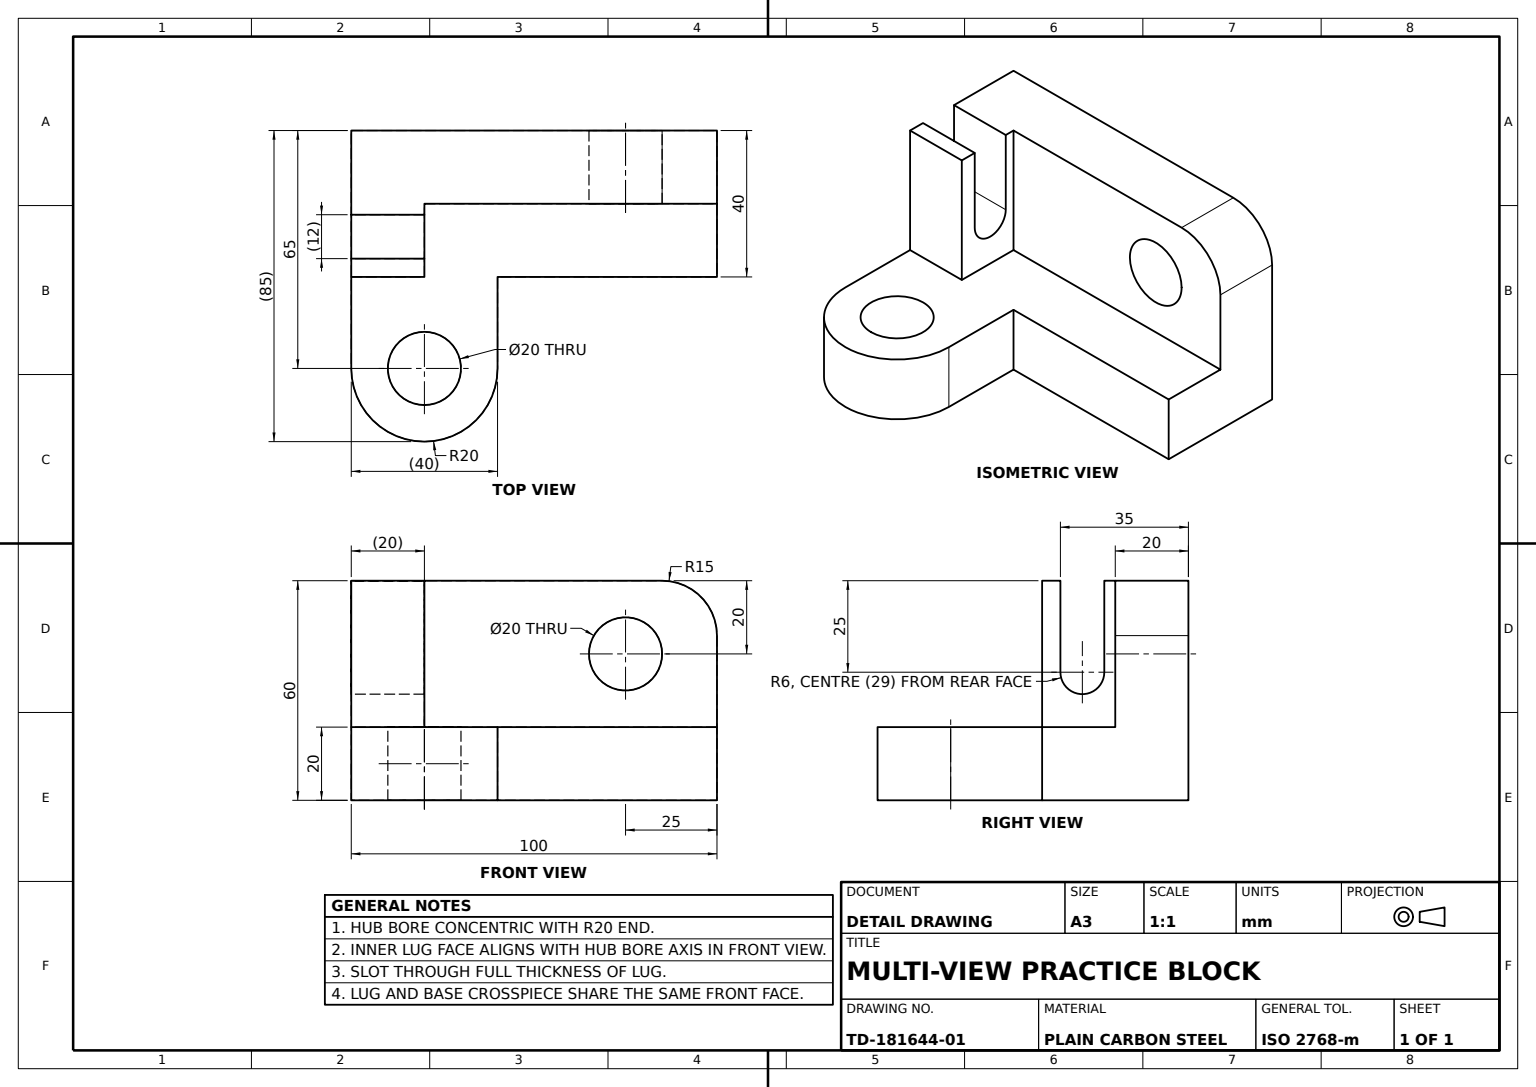
SolidWorks part; units mm, degrees
material "Plain Carbon Steel"
ref_plane "Front Plane" through (0, 0, 0) normal (0, 0, 1) x (1, 0, 0)
ref_plane "Top Plane" through (0, 0, 0) normal (0, 1, 0) x (1, 0, 0)
ref_plane "Right Plane" through (0, 0, 0) normal (1, 0, 0) x (0, 0, -1)
sketch "Base Block Profile" plane through (0, 0, 0) normal (0, 0, 1) x (1, 0, 0)
  line L0 (0, 0) -> (-85, 0)
  line L1 (-100, 60) -> (0, 60)
  line L2 (0, 60) -> (0, 0)
  line L3 (-100, 15) -> (-100, 60)
  arc A0 (-100, 15) -> (-85, 0) centre (-85, 15) ccw
  dimension "D1" = 30
  dimension "D3" = 15
  dimension "D2" = 100
  dimension "D4" = 60
extrude "Base Block" add sketch "Base Block Profile" along normal blind 20
sketch "Hub Boss Profile" plane through (0, 0, 0) normal (1, 0, 0) x (0, 0, -1)
  line L0 (-20, 0) -> (-20, 40)
  line L1 (-20, 0) -> (-20, 60) construction
  line L2 (-20, 40) -> (-40, 40)
  line L3 (-40, 40) -> (-40, 0)
  line L4 (-40, 0) -> (-35, 0)
  line L5 (-20, 0) -> (-23, 0)
  line L6 (-23, 0) -> (-23, 25)
  line L8 (-35, 25) -> (-35, 0)
  line L9 (0, 0) -> (0, 60) construction
  line L10 (-20, 60) -> (0, 60) construction
  arc A0 (-23, 25) -> (-35, 25) centre (-29, 25) ccw
  dimension "D1" = 12
  dimension "D2" = 6
  dimension "D3" = 29
  dimension "D4" = 40
  dimension "D5" = 20
  dimension "D6" = 35
extrude "Hub Boss" add sketch "Hub Boss Profile" against normal blind 20
sketch "Leg Profile" plane through (0, 60, 0) normal (0, 1, 0) x (1, 0, 0)
  line L0 (-100, -20) -> (-100, -40)
  line L1 (-100, -40) -> (-40, -40)
  line L2 (-40, -40) -> (-40, -20)
  line L3 (0, -20) -> (-100, -20) construction
  line L4 (-40, -20) -> (-100, -20)
  line L5 (-100, -20) -> (-100, 0) construction
  line L6 (0, 0) -> (-100, 0) construction
  dimension "D1" = 60
  dimension "D2" = 40
extrude "Leg" add sketch "Leg Profile" against normal blind 20
sketch "Top Arm Profile" plane through (0, 60, 0) normal (0, 1, 0) x (1, 0, 0)
  line L0 (-40, -20) -> (0, -20)
  line L1 (0, -20) -> (0, -65)
  line L3 (-40, -65) -> (-40, -20)
  line L5 (0, 0) -> (-100, 0) construction
  arc A0 (-40, -65) -> (0, -65) centre (-20, -65) ccw
  dimension "D1" = 40
  dimension "D2" = 65
extrude "Top Arm" add sketch "Top Arm Profile" against normal blind 20
sketch "Hub Bore Sketch" plane through (0, 40, 0) normal (0, -1, 0) x (1, 0, 0)
  circle A0 centre (-20, 65) radius 10
  dimension "D1" = 20
  dimension "D2" = 20
extrude "Hub Bore Cut" cut sketch "Hub Bore Sketch" against normal blind 20
sketch "Leg Slot Sketch" plane through (0, 0, 20) normal (0, 0, 1) x (1, 0, 0)
  line L0 (-100, 40) -> (-100, 15) construction
  line L2 (-85, 0) -> (-20, 0) construction
  circle A0 centre (-75, 20) radius 10
  dimension "D1" = 20
  dimension "D4" = 20
  dimension "D2" = 25
  dimension "D3" = 20
extrude "Leg Slot Cut" cut sketch "Leg Slot Sketch" against normal blind 20
